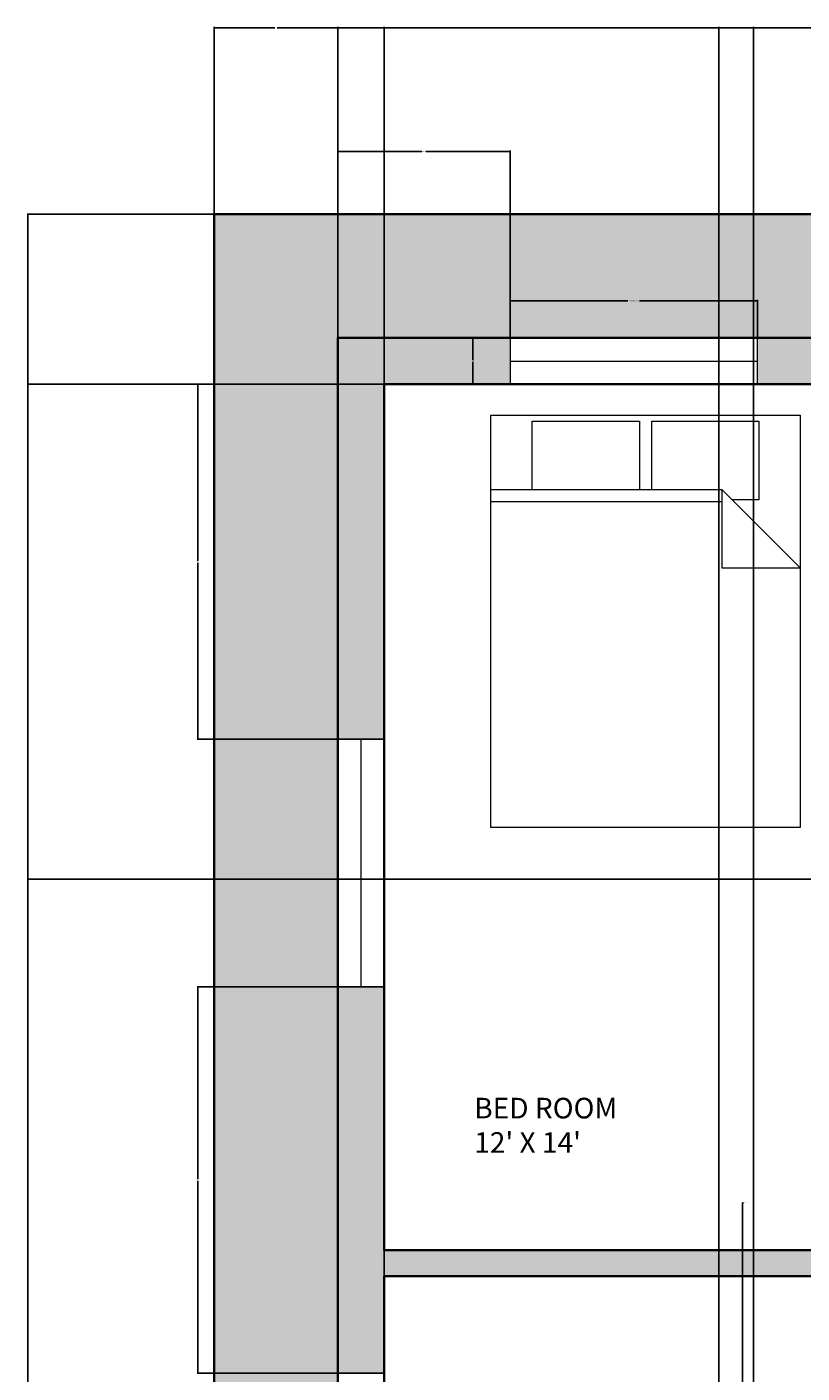
# Model space of a CAD drawing. Units: inches. Extents: x -7 to 546, y -27 to 766.
# Tile 6 of 9: x -7 to 143, y 505 to 766. Entities that reach past the tile are written whole.
import ezdxf

# ---------------------------------------------------------------- set-up
doc = ezdxf.new("R2010")
doc.units = ezdxf.units.IN
doc.header["$MEASUREMENT"] = 0
for name, color, linetype, lineweight in [('A-ANNO-DIMS', 2, 'Continuous', 18), ('A-AREA-IDEN', 7, 'Continuous', 18), ('A-WALL', 7, 'Continuous', 35), ('C-PROP', 7, 'Continuous', 35), ('furniture', 220, 'Continuous', 18), ('window', 30, 'Continuous', 20)]:
    doc.layers.add(name, color=color, linetype=linetype, lineweight=lineweight)
doc.layers.add('A-WALL-PATT', color=251, linetype='Continuous', lineweight=13, true_color=0x636466)
doc.layers.add('L-PLNT-PATT', color=85, linetype='Continuous', lineweight=13, true_color=0x58ba48)
doc.styles.get("Standard").update_dxf_attribs({"font": 'arial.ttf'})
doc.dimstyles.get("Standard").update_dxf_attribs({"dimtxt": 0.18, "dimasz": 0.18, "dimexe": 0.18, "dimexo": 0.0625, "dimgap": 0.09, "dimtad": 0, "dimtih": 1, "dimtoh": 1, "dimdec": 4, "dimzin": 0, "dimdsep": 46, "dimtxsty": 'Standard', "dimcen": 0.09, "dimadec": 0, "dimazin": 0, "dimtfac": 1, "dimtdec": 4, "dimtofl": 0, "dimtmove": 0, "dimatfit": 3, "dimfxl": 1, "dimtolj": 1, "dimtzin": 0, "dimarcsym": 0})

# ---------------------------------------------------------------- blocks, each defined once
blk = doc.blocks.new('Bed - Queen')
for p, q in [((0, -80.00003), (0, 0)), ((0, 0), (59.99999, 0)), ((59.99999, 0), (59.99999, -80.00003)), ((7.99999, -1.2), (28.79998, -1.2)), ((7.99999, -14.4), (7.99999, -1.2)), ((28.79998, -1.2), (28.79998, -14.4)), ((31.19999, -1.2), (51.99999, -1.2)), ((31.19999, -14.4), (31.19999, -1.2)), ((51.99999, -1.2), (51.99999, -16.4)), ((0, -14.4), (44.8, -14.4)), ((59.99999, -29.6), (44.8, -14.4)), ((44.8, -14.4), (44.8, -29.6)), ((44.8, -16.8), (0, -16.8)), ((51.99999, -16.4), (46.79936, -16.4)), ((44.8, -29.6), (59.99999, -29.6)), ((59.99999, -80.00003), (0, -80.00003))]:
    blk.add_line(p, q)
blk = doc.blocks.new('WIN-48IN')
for p, q in [((0, 9), (0, 0)), ((48, 9), (0, 9)), ((0, 9), (0, 4.5)), ((48, 0), (48, 9)), ((0, 4.5), (48, 4.5)), ((0, 0), (48, 0))]:
    blk.add_line(p, q)
blk = doc.blocks.new('*D14')
at = {"layer": 'A-ANNO-DIMS', "color": 0, "lineweight": -2, "transparency": 16777216}
for p, q in [((86.69, 705.81), (86.69, 713.12)), ((86.87, 712.94), (109.57, 712.94)), ((134.51, 712.94), (111.81, 712.94)), ((134.69, 705.81), (134.69, 713.12))]:
    blk.add_line(p, q, dxfattribs=at)
at = {"layer": 'A-ANNO-DIMS', "color": 0, "transparency": 16777216}
for points in [[(86.87, 712.97), (86.87, 712.91), (86.69, 712.94)], [(134.51, 712.97), (134.51, 712.91), (134.69, 712.94)]]:
    blk.add_solid(points, dxfattribs=at)
at = {"layer": 'Defpoints', "color": 0, "transparency": 16777216}
for p in [(134.69, 712.94), (86.69, 705.74), (134.69, 705.74)]:
    blk.add_point(p, dxfattribs=at)
at = {"layer": 'A-ANNO-DIMS', "color": 0, "transparency": 16777216, "insert": (110.69, 712.94), "char_height": 0.18, "attachment_point": 5}
blk.add_mtext('\\A1;WINDOW 48 TYP.', dxfattribs=at)
blk = doc.blocks.new('*D15')
at = {"layer": 'A-ANNO-DIMS', "color": 0, "lineweight": -2, "transparency": 16777216}
for p, q in [((86.63, 705.74), (79.31, 705.74)), ((79.49, 705.56), (79.49, 701.43)), ((79.49, 696.92), (79.49, 701.06)), ((86.63, 696.74), (79.31, 696.74))]:
    blk.add_line(p, q, dxfattribs=at)
at = {"layer": 'A-ANNO-DIMS', "color": 0, "transparency": 16777216}
for points in [[(79.46, 705.56), (79.52, 705.56), (79.49, 705.74)], [(79.46, 696.92), (79.52, 696.92), (79.49, 696.74)]]:
    blk.add_solid(points, dxfattribs=at)
at = {"layer": 'Defpoints', "color": 0, "transparency": 16777216}
for p in [(79.49, 705.74), (86.69, 705.74), (86.69, 696.74)]:
    blk.add_point(p, dxfattribs=at)
at = {"layer": 'A-ANNO-DIMS', "color": 0, "transparency": 16777216, "insert": (79.49, 701.24), "char_height": 0.18, "attachment_point": 5}
blk.add_mtext('\\A1;9 TYP.', dxfattribs=at)
blk = doc.blocks.new('*D31')
at = {"layer": 'A-ANNO-DIMS', "color": 0, "lineweight": -2, "transparency": 16777216}
for p, q in [((29.17, 729.74), (-7.07, 729.74)), ((-6.89, 729.56), (-6.89, 369.93)), ((-6.89, 9.92), (-6.89, 369.56)), ((29.17, 9.74), (-7.07, 9.74))]:
    blk.add_line(p, q, dxfattribs=at)
at = {"layer": 'A-ANNO-DIMS', "color": 0, "transparency": 16777216}
for points in [[(-6.92, 729.56), (-6.86, 729.56), (-6.89, 729.74)], [(-6.92, 9.92), (-6.86, 9.92), (-6.89, 9.74)]]:
    blk.add_solid(points, dxfattribs=at)
at = {"layer": 'Defpoints', "color": 0, "transparency": 16777216}
for p in [(-6.89, 729.74), (29.23, 729.74), (29.23, 9.74)]:
    blk.add_point(p, dxfattribs=at)
at = {"layer": 'A-ANNO-DIMS', "color": 0, "transparency": 16777216, "insert": (-6.89, 369.74), "char_height": 0.18, "attachment_point": 5}
blk.add_mtext('\\A1;720', dxfattribs=at)
blk = doc.blocks.new('*D32')
at = {"layer": 'A-ANNO-DIMS', "color": 0, "lineweight": -2, "transparency": 16777216}
for p, q in [((53.23, 705.81), (53.23, 766.05)), ((53.41, 765.87), (268.94, 765.87)), ((485.05, 765.87), (269.52, 765.87)), ((485.23, 705.81), (485.23, 766.05))]:
    blk.add_line(p, q, dxfattribs=at)
at = {"layer": 'A-ANNO-DIMS', "color": 0, "transparency": 16777216}
for points in [[(53.41, 765.9), (53.41, 765.84), (53.23, 765.87)], [(485.05, 765.9), (485.05, 765.84), (485.23, 765.87)]]:
    blk.add_solid(points, dxfattribs=at)
at = {"layer": 'Defpoints', "color": 0, "transparency": 16777216}
for p in [(485.23, 765.87), (53.23, 705.74), (485.23, 705.74)]:
    blk.add_point(p, dxfattribs=at)
at = {"layer": 'A-ANNO-DIMS', "color": 0, "transparency": 16777216, "insert": (269.23, 765.87), "char_height": 0.18, "attachment_point": 5}
blk.add_mtext('\\A1;432', dxfattribs=at)
blk = doc.blocks.new('*D34')
at = {"layer": 'A-ANNO-DIMS', "color": 0, "lineweight": -2, "transparency": 16777216}
for p, q in [((29.23, 729.81), (29.23, 766.05)), ((29.41, 765.87), (41.01, 765.87)), ((53.05, 765.87), (41.45, 765.87)), ((53.23, 705.81), (53.23, 766.05))]:
    blk.add_line(p, q, dxfattribs=at)
at = {"layer": 'A-ANNO-DIMS', "color": 0, "transparency": 16777216}
for points in [[(29.41, 765.9), (29.41, 765.84), (29.23, 765.87)], [(53.05, 765.9), (53.05, 765.84), (53.23, 765.87)]]:
    blk.add_solid(points, dxfattribs=at)
at = {"layer": 'Defpoints', "color": 0, "transparency": 16777216}
for p in [(53.23, 765.87), (29.23, 729.74), (53.23, 705.74)]:
    blk.add_point(p, dxfattribs=at)
at = {"layer": 'A-ANNO-DIMS', "color": 0, "transparency": 16777216, "insert": (41.23, 765.87), "char_height": 0.18, "attachment_point": 5}
blk.add_mtext('\\A1;24', dxfattribs=at)
blk = doc.blocks.new('*D38')
at = {"layer": 'A-ANNO-DIMS', "color": 0, "lineweight": -2, "transparency": 16777216}
for p, q in [((211.17, 696.74), (-7.07, 696.74)), ((-6.89, 696.56), (-6.89, 648.93)), ((-6.89, 600.92), (-6.89, 648.56)), ((211.17, 600.74), (-7.07, 600.74))]:
    blk.add_line(p, q, dxfattribs=at)
at = {"layer": 'A-ANNO-DIMS', "color": 0, "transparency": 16777216}
for points in [[(-6.92, 696.56), (-6.86, 696.56), (-6.89, 696.74)], [(-6.92, 600.92), (-6.86, 600.92), (-6.89, 600.74)]]:
    blk.add_solid(points, dxfattribs=at)
at = {"layer": 'Defpoints', "color": 0, "transparency": 16777216}
for p in [(211.23, 696.74), (-6.89, 600.74), (211.23, 600.74)]:
    blk.add_point(p, dxfattribs=at)
at = {"layer": 'A-ANNO-DIMS', "color": 0, "transparency": 16777216, "insert": (-6.89, 648.74), "char_height": 0.18, "attachment_point": 5}
blk.add_mtext('\\A1;96', dxfattribs=at)
blk = doc.blocks.new('*D53')
at = {"layer": 'A-ANNO-DIMS', "color": 0, "lineweight": -2, "transparency": 16777216}
for p, q in [((133.93, 124.01), (133.93, 766.05)), ((134.11, 765.87), (181.71, 765.87)), ((229.75, 765.87), (182.15, 765.87)), ((229.93, 124.01), (229.93, 766.05))]:
    blk.add_line(p, q, dxfattribs=at)
at = {"layer": 'A-ANNO-DIMS', "color": 0, "transparency": 16777216}
for points in [[(134.11, 765.9), (134.11, 765.84), (133.93, 765.87)], [(229.75, 765.9), (229.75, 765.84), (229.93, 765.87)]]:
    blk.add_solid(points, dxfattribs=at)
at = {"layer": 'Defpoints', "color": 0, "transparency": 16777216}
for p in [(229.93, 765.87), (133.93, 123.94), (229.93, 123.94)]:
    blk.add_point(p, dxfattribs=at)
at = {"layer": 'A-ANNO-DIMS', "color": 0, "transparency": 16777216, "insert": (181.93, 765.87), "char_height": 0.18, "attachment_point": 5}
blk.add_mtext('\\A1;96', dxfattribs=at)
blk = doc.blocks.new('*D68')
at = {"layer": 'A-ANNO-DIMS', "color": 0, "lineweight": -2, "transparency": 16777216}
for p, q in [((133.93, 100.01), (133.93, 766.05)), ((134.11, 765.87), (149.71, 765.87)), ((165.75, 765.87), (150.15, 765.87)), ((165.93, 104.01), (165.93, 766.05))]:
    blk.add_line(p, q, dxfattribs=at)
at = {"layer": 'A-ANNO-DIMS', "color": 0, "transparency": 16777216}
for points in [[(134.11, 765.9), (134.11, 765.84), (133.93, 765.87)], [(165.75, 765.9), (165.75, 765.84), (165.93, 765.87)]]:
    blk.add_solid(points, dxfattribs=at)
at = {"layer": 'Defpoints', "color": 0, "transparency": 16777216}
for p in [(165.93, 765.87), (165.93, 103.94), (133.93, 99.94)]:
    blk.add_point(p, dxfattribs=at)
at = {"layer": 'A-ANNO-DIMS', "color": 0, "transparency": 16777216, "insert": (149.93, 765.87), "char_height": 0.18, "attachment_point": 5}
blk.add_mtext('\\A1;32', dxfattribs=at)
blk = doc.blocks.new('*D71')
at = {"layer": 'A-ANNO-DIMS', "color": 0, "lineweight": -2, "transparency": 16777216}
for p, q in [((53.23, 705.81), (53.23, 742.05)), ((53.41, 741.87), (69.57, 741.87)), ((86.51, 741.87), (70.35, 741.87)), ((86.69, 705.81), (86.69, 742.05))]:
    blk.add_line(p, q, dxfattribs=at)
at = {"layer": 'A-ANNO-DIMS', "color": 0, "transparency": 16777216}
for points in [[(53.41, 741.9), (53.41, 741.84), (53.23, 741.87)], [(86.51, 741.9), (86.51, 741.84), (86.69, 741.87)]]:
    blk.add_solid(points, dxfattribs=at)
at = {"layer": 'Defpoints', "color": 0, "transparency": 16777216}
for p in [(86.69, 741.87), (53.23, 705.74), (86.69, 705.74)]:
    blk.add_point(p, dxfattribs=at)
at = {"layer": 'A-ANNO-DIMS', "color": 0, "transparency": 16777216, "insert": (69.96, 741.87), "char_height": 0.18, "attachment_point": 5}
blk.add_mtext('\\A1;33.46', dxfattribs=at)
blk = doc.blocks.new('*D72')
at = {"layer": 'A-ANNO-DIMS', "color": 0, "lineweight": -2, "transparency": 16777216}
for p, q in [((62.16, 579.86), (25.92, 579.86)), ((26.1, 579.68), (26.1, 542.58)), ((26.1, 505.11), (26.1, 542.21)), ((62.16, 504.93), (25.92, 504.93))]:
    blk.add_line(p, q, dxfattribs=at)
at = {"layer": 'A-ANNO-DIMS', "color": 0, "transparency": 16777216}
for points in [[(26.07, 579.68), (26.13, 579.68), (26.1, 579.86)], [(26.07, 505.11), (26.13, 505.11), (26.1, 504.93)]]:
    blk.add_solid(points, dxfattribs=at)
at = {"layer": 'Defpoints', "color": 0, "transparency": 16777216}
for p in [(26.1, 579.86), (62.23, 579.86), (62.23, 504.93)]:
    blk.add_point(p, dxfattribs=at)
at = {"layer": 'A-ANNO-DIMS', "color": 0, "transparency": 16777216, "insert": (26.1, 542.4), "char_height": 0.18, "attachment_point": 5}
blk.add_mtext('\\A1;74.94', dxfattribs=at)
blk = doc.blocks.new('*D74')
at = {"layer": 'A-ANNO-DIMS', "color": 0, "lineweight": -2, "transparency": 16777216}
for p, q in [((62.17, 696.74), (25.93, 696.75)), ((26.11, 696.57), (26.1, 662.49)), ((26.1, 628.05), (26.1, 662.12)), ((62.16, 627.86), (25.92, 627.87))]:
    blk.add_line(p, q, dxfattribs=at)
at = {"layer": 'A-ANNO-DIMS', "color": 0, "transparency": 16777216}
for points in [[(26.08, 696.57), (26.14, 696.57), (26.11, 696.75)], [(26.07, 628.05), (26.13, 628.05), (26.1, 627.87)]]:
    blk.add_solid(points, dxfattribs=at)
at = {"layer": 'Defpoints', "color": 0, "transparency": 16777216}
for p in [(26.11, 696.75), (62.23, 696.74), (62.23, 627.86)]:
    blk.add_point(p, dxfattribs=at)
at = {"layer": 'A-ANNO-DIMS', "color": 0, "transparency": 16777216, "insert": (26.1, 662.31), "char_height": 0.18, "attachment_point": 5}
blk.add_mtext('\\A1;68.88', dxfattribs=at)
blk = doc.blocks.new('*D81')
at = {"layer": 'A-ANNO-DIMS', "color": 0, "lineweight": -2, "transparency": 16777216}
for p, q in [((62.23, 240.81), (62.23, 766.05)), ((62.41, 765.87), (194.44, 765.87)), ((327.05, 765.87), (195.02, 765.87)), ((327.23, 234.81), (327.23, 766.05))]:
    blk.add_line(p, q, dxfattribs=at)
at = {"layer": 'A-ANNO-DIMS', "color": 0, "transparency": 16777216}
for points in [[(62.41, 765.9), (62.41, 765.84), (62.23, 765.87)], [(327.05, 765.9), (327.05, 765.84), (327.23, 765.87)]]:
    blk.add_solid(points, dxfattribs=at)
at = {"layer": 'Defpoints', "color": 0, "transparency": 16777216}
for p in [(327.23, 765.87), (62.23, 240.74), (327.23, 234.74)]:
    blk.add_point(p, dxfattribs=at)
at = {"layer": 'A-ANNO-DIMS', "color": 0, "transparency": 16777216, "insert": (194.73, 765.87), "char_height": 0.18, "attachment_point": 5}
blk.add_mtext('\\A1;265', dxfattribs=at)
blk = doc.blocks.new('*D83')
at = {"layer": 'A-ANNO-DIMS', "color": 0, "lineweight": -2, "transparency": 16777216}
for p, q in [((127.23, 91.81), (127.23, 766.05)), ((127.41, 765.87), (130.18, 765.87)), ((133.75, 765.87), (130.97, 765.87)), ((133.93, 100.01), (133.93, 766.05))]:
    blk.add_line(p, q, dxfattribs=at)
at = {"layer": 'A-ANNO-DIMS', "color": 0, "transparency": 16777216}
for points in [[(127.41, 765.9), (127.41, 765.84), (127.23, 765.87)], [(133.75, 765.9), (133.75, 765.84), (133.93, 765.87)]]:
    blk.add_solid(points, dxfattribs=at)
at = {"layer": 'Defpoints', "color": 0, "transparency": 16777216}
for p in [(133.93, 765.87), (133.93, 99.94), (127.23, 91.74)]:
    blk.add_point(p, dxfattribs=at)
at = {"layer": 'A-ANNO-DIMS', "color": 0, "transparency": 16777216, "insert": (130.58, 765.87), "char_height": 0.18, "attachment_point": 5}
blk.add_mtext('\\A1;6.695', dxfattribs=at)
blk = doc.blocks.new('*D89')
at = {"layer": 'A-ANNO-DIMS', "color": 0, "lineweight": -2, "transparency": 16777216}
for p, q in [((131.97, 537.98), (131.79, 537.98)), ((131.79, 537.98), (131.79, 465.44)), ((131.7, 344.07), (131.88, 344.07)), ((131.79, 343.98), (131.79, 344.16))]:
    blk.add_line(p, q, dxfattribs=at)
at = {"layer": 'A-ANNO-DIMS', "color": 0, "transparency": 16777216}
blk.add_solid([(131.76, 465.44), (131.82, 465.44), (131.79, 465.26)], dxfattribs=at)
at = {"layer": 'Defpoints', "color": 0, "transparency": 16777216}
for p in [(131.79, 465.26), (131.79, 344.07)]:
    blk.add_point(p, dxfattribs=at)
at = {"layer": 'A-ANNO-DIMS', "color": 0, "transparency": 16777216, "insert": (132.65, 537.98), "char_height": 0.18, "attachment_point": 5}
blk.add_mtext('\\A1;3X R121.2', dxfattribs=at)

msp = doc.modelspace()

# ---------------------------------------------------------------- hatches: boundary and pattern name
at = {"layer": 'A-WALL-PATT'}
h = msp.add_hatch(color=256, dxfattribs=at)
h.dxf.hatch_style = 1
h.paths.add_polyline_path([(62.2319, 696.744), (86.6896, 696.744), (86.6896, 705.744), (53.2319, 705.744), (53.2319, 627.8642), (57.7271, 627.8642), (62.2319, 627.8642)])
h.paths.add_polyline_path([(229.7414, 705.744), (134.6896, 705.744), (134.6896, 696.744), (206.2319, 696.744), (206.2319, 567.744), (211.2319, 567.744), (211.2319, 595.744), (214.2319, 595.744), (214.2319, 600.744), (211.2319, 600.744), (211.2319, 696.744), (229.7414, 696.744)])
h.paths.add_polyline_path([(293.8423, 705.744), (253.7414, 705.744), (253.7414, 696.744), (274.2319, 696.744), (274.2319, 600.744), (279.2319, 600.744), (279.2319, 696.744), (293.8423, 696.744)])
h.paths.add_polyline_path([(393.9743, 705.744), (317.8423, 705.744), (317.8423, 696.744), (327.2319, 696.744), (327.2319, 651.744), (332.2319, 651.744), (332.2319, 696.744), (393.9743, 696.744)])
h.paths.add_polyline_path([(485.2319, 705.744), (441.9743, 705.744), (441.9743, 696.744), (476.2319, 696.744), (476.2319, 663.6898), (480.7319, 663.6898), (485.2319, 663.6898)])
h.paths.add_polyline_path([(485.2319, 615.6898), (476.2319, 615.6898), (476.2319, 528.744), (332.2319, 528.744), (332.2319, 531.744), (327.2319, 531.744), (327.2319, 523.744), (375.2319, 523.744), (375.2319, 427.744), (327.2319, 427.744), (327.2319, 419.744), (332.2319, 419.744), (332.2319, 422.744), (413.089, 422.744), (413.089, 427.744), (380.2319, 427.744), (380.2319, 523.744), (476.2319, 523.744), (476.2319, 490.9334), (485.2319, 490.9334)])
h.paths.add_polyline_path([(485.2319, 466.9334), (476.2319, 466.9334), (476.2319, 370.0932), (480.7319, 370.0932), (485.2319, 370.0932)])
h.paths.add_polyline_path([(485.2319, 322.0932), (476.2319, 322.0932), (476.2319, 278.744), (332.2319, 278.744), (332.2319, 383.744), (327.2319, 383.744), (327.2319, 273.744), (327.2319, 270.744), (332.2319, 270.744), (332.2319, 273.744), (476.2319, 273.744), (476.2319, 201.0338), (480.7319, 201.0338), (485.2319, 201.0338)])
h.paths.add_polyline_path([(485.2319, 153.0338), (476.2319, 153.0338), (476.2319, 42.744), (461.2319, 42.744), (461.2319, 33.744), (485.2319, 33.744)])
h.paths.add_polyline_path([(332.2319, 234.744), (327.2319, 234.744), (327.2319, 160.744), (315.2319, 160.744), (315.2319, 151.744), (327.2319, 151.744), (327.2319, 33.744), (332.2319, 33.744)])
h.paths.add_polyline_path([(252.2319, 151.744), (258.4464, 151.744), (264.2319, 151.744), (264.2319, 160.744), (252.2319, 160.744), (252.2319, 172.744), (247.2319, 172.744), (247.2319, 91.744), (127.2319, 91.744), (127.2319, 196.744), (122.2319, 196.744), (122.2319, 91.744), (62.2319, 91.744), (62.2319, 126.1124), (53.2319, 126.1124), (53.2319, 9.744), (62.2319, 9.744), (62.2319, 86.744), (247.2319, 86.744), (247.2319, 33.744), (252.2319, 33.744), (252.2319, 53.744)])
h.paths.add_polyline_path([(62.2319, 235.744), (122.2319, 235.744), (122.2319, 232.744), (127.2319, 232.744), (127.2319, 235.744), (247.2319, 235.744), (247.2319, 220.744), (252.2319, 220.744), (252.2319, 240.744), (250.6678, 240.744), (247.2319, 240.744), (62.2319, 240.744), (62.2319, 322.0932), (53.2319, 322.0932), (53.2319, 174.1124), (57.7271, 174.1124), (62.2319, 174.1124)])
h = msp.add_hatch(color=256, dxfattribs=at)
h.dxf.hatch_style = 1
h.paths.add_polyline_path([(62.2319, 456.9275), (53.2319, 456.9275), (53.2319, 370.0932), (57.7271, 370.0932), (62.2319, 370.0932)])
h.paths.add_polyline_path([(62.2319, 579.8642), (53.2319, 579.8642), (53.2319, 504.9275), (57.7271, 504.9275), (62.2319, 504.9275), (62.2319, 523.744), (211.2319, 523.744), (211.2319, 531.744), (206.2319, 531.744), (206.2319, 528.744), (62.2319, 528.744)])
at = {"layer": 'L-PLNT-PATT'}
h = msp.add_hatch(color=256, dxfattribs=at)
h.dxf.hatch_style = 1
h.paths.add_polyline_path([(509.2319, 729.744), (29.2319, 729.744), (29.2319, 9.744), (53.2319, 9.744), (53.2319, 705.744), (485.2319, 705.744), (485.2319, 33.744), (461.2319, 33.744), (461.2319, 9.744), (509.2319, 9.744)])

# ---------------------------------------------------------------- linework, layer by layer
at = {"layer": 'A-WALL'}
for p, q in [((206.2319, 696.744), (62.2319, 696.744)), ((62.2319, 696.744), (62.2319, 528.744)), ((206.2319, 528.744), (62.2319, 528.744)), ((211.2319, 523.744), (62.2319, 523.744)), ((62.2319, 523.744), (62.2319, 240.744))]:
    msp.add_line(p, q, dxfattribs=at)
msp.add_lwpolyline([(461.2319, 33.744), (485.2319, 33.744), (485.2319, 705.744), (53.2319, 705.744), (53.2319, 9.744)], dxfattribs=at)
at = {"layer": 'C-PROP'}
msp.add_lwpolyline([(29.2319, 9.744), (509.2319, 9.744), (509.2319, 729.744), (29.2319, 729.744)], close=True, dxfattribs=at)

# ---------------------------------------------------------------- block references
at = {"layer": 'furniture'}
msp.add_blockref('Bed - Queen', (82.9819, 690.748), dxfattribs=at)
at = {"layer": 'window'}
msp.add_blockref('WIN-48IN', (86.69, 696.744), dxfattribs=at)
at = {"layer": 'window', "extrusion": (0, 0, -1), "zscale": -1, "rotation": 270}
msp.add_blockref('WIN-48IN', (-62.227, 627.8638), dxfattribs=at)

# ---------------------------------------------------------------- texts
at = {"layer": 'A-AREA-IDEN', "insert": (79.7254, 558.3228), "char_height": 4, "attachment_point": 1}
msp.add_mtext_dynamic_manual_height_columns("BED ROOM\\P12' X 14'", width=80.777321, gutter_width=1, heights=[0], dxfattribs=at)

# ---------------------------------------------------------------- dimensions: what is measured, and where the dimension line sits
at = {"layer": 'A-ANNO-DIMS'}
for base, p1, p2, override, picture, middle in [((53.2319, 765.869), (29.2319, 729.744), (53.2319, 705.744), {"dimdec": 0, "dimlfac": 1, "dimrnd": 0, "dimzin": 0, "dimdsep": 46, "dimlunit": 2}, '*D34', (41.2319, 765.869)), ((485.2319, 765.869), (53.2319, 705.744), (485.2319, 705.744), {"dimdec": 0, "dimlfac": 1, "dimrnd": 0, "dimzin": 0, "dimdsep": 46, "dimlunit": 2}, '*D32', (269.2319, 765.869)), ((327.2319, 765.869), (62.2319, 240.744), (327.2319, 234.744), {"dimdec": 0, "dimlfac": 1, "dimrnd": 0, "dimzin": 0, "dimdsep": 46, "dimlunit": 2}, '*D81', (194.7319, 765.869)), ((133.9271, 765.869), (127.2319, 91.744), (133.9271, 99.9426), {"dimdec": 3, "dimlfac": 1, "dimrnd": 0, "dimzin": 0, "dimdsep": 46, "dimlunit": 2}, '*D83', (130.5795, 765.869)), ((229.9271, 765.869), (133.9271, 123.9426), (229.9271, 123.9426), {"dimdec": 0, "dimlfac": 1, "dimrnd": 0, "dimzin": 0, "dimdsep": 46, "dimlunit": 2}, '*D53', (181.9271, 765.869)), ((165.9271, 765.869), (133.9271, 99.9426), (165.9271, 103.9426), {"dimdec": 0, "dimlfac": 1, "dimrnd": 0, "dimzin": 0, "dimdsep": 46, "dimlunit": 2}, '*D68', (149.9271, 765.869))]:
    dim = msp.add_linear_dim(base=base, p1=p1, p2=p2, dimstyle='Standard', override=override, dxfattribs=at)
    dim.commit()
    dim.dimension.update_dxf_attribs({"geometry": picture, "text_midpoint": middle})
for base, p1, p2, angle, override, picture, middle in [((86.6896, 741.869), (53.2319, 705.744), (86.6896, 705.744), 0, {"dimdec": 2, "dimlfac": 1, "dimrnd": 0, "dimzin": 0, "dimdsep": 46, "dimlunit": 2}, '*D71', (69.9608, 741.869)), ((-6.8931, 729.744), (29.2319, 9.744), (29.2319, 729.744), 90, {"dimdec": 0, "dimlfac": 1, "dimrnd": 0, "dimzin": 0, "dimdsep": 46, "dimlunit": 2}, '*D31', (-6.8931, 369.744)), ((-6.8931, 600.744), (211.2319, 696.744), (211.2319, 600.744), 90, {"dimdec": 0, "dimlfac": 1, "dimrnd": 0, "dimzin": 0, "dimdsep": 46, "dimlunit": 2}, '*D38', (-6.8931, 648.744)), ((26.1069, 696.7465), (62.2271, 627.8642), (62.2319, 696.744), 89.995961, {"dimdec": 2, "dimlfac": 1, "dimrnd": 0, "dimzin": 0, "dimdsep": 46, "dimlunit": 2}, '*D74', (26.1045, 662.3066)), ((26.1021, 579.8642), (62.2271, 504.9275), (62.2271, 579.8642), 90, {"dimdec": 2, "dimlfac": 1, "dimrnd": 0, "dimzin": 0, "dimdsep": 46, "dimlunit": 2}, '*D72', (26.1021, 542.3958))]:
    dim = msp.add_linear_dim(base=base, p1=p1, p2=p2, angle=angle, dimstyle='Standard', override=override, dxfattribs=at)
    dim.commit()
    dim.dimension.update_dxf_attribs({"geometry": picture, "text_midpoint": middle})
dim = msp.add_linear_dim(base=(134.6896, 712.944), p1=(86.6896, 705.744), p2=(134.6896, 705.744), text='WINDOW <> TYP.', dimstyle='Standard', override={"dimdec": 0, "dimlfac": 1, "dimrnd": 0, "dimzin": 0, "dimdsep": 46, "dimlunit": 2}, dxfattribs=at)
dim.commit()
dim.dimension.update_dxf_attribs({"geometry": '*D14', "text_midpoint": (110.6896, 712.944)})
dim = msp.add_linear_dim(base=(79.4896, 705.744), p1=(86.6896, 696.744), p2=(86.6896, 705.744), angle=90, text='<> TYP.', dimstyle='Standard', override={"dimdec": 0, "dimlfac": 1, "dimrnd": 0, "dimzin": 0, "dimdsep": 46, "dimlunit": 2}, dxfattribs=at)
dim.commit()
dim.dimension.update_dxf_attribs({"geometry": '*D15', "text_midpoint": (79.4896, 701.244)})
dim = msp.add_radius_dim(center=(131.7927, 344.066), mpoint=(131.793, 465.2628), text='3X <>', dimstyle='Standard', override={"dimdec": 1, "dimlfac": 1, "dimrnd": 0, "dimzin": 0, "dimdsep": 46, "dimlunit": 2}, dxfattribs=at)
dim.commit()
dim.dimension.update_dxf_attribs({"geometry": '*D89', "text_midpoint": (132.6454, 537.9809), "dimtype": 164})

doc.saveas('drawing.dxf')
